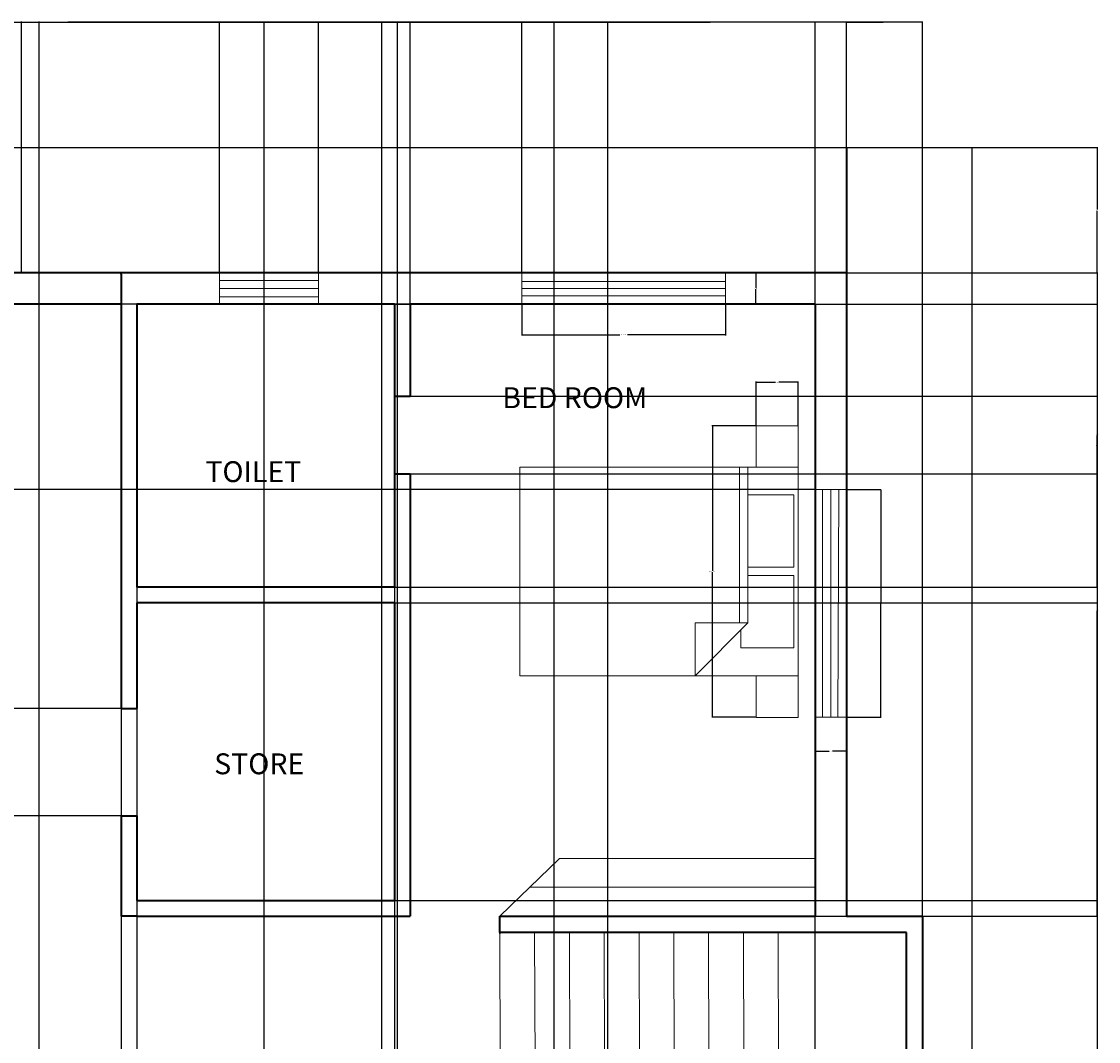
# Model space of a CAD drawing. Units: inches. Extents: x 2621 to 3621, y 1701 to 2465.
# Tile 4 of 6: x 2780 to 3090, y 2169 to 2462. Entities that reach past the tile are written whole.
import ezdxf

# ---------------------------------------------------------------- set-up
doc = ezdxf.new("R2010")
doc.units = ezdxf.units.IN
for name, color, linetype, lineweight in [('A-ANNO-DIMS', 2, 'Continuous', 18), ('A-AREA-IDEN', 7, 'Continuous', 18), ('A-FLOR-CASE', 32, 'Continuous', 18), ('A-FLOR-STRS', 30, 'Continuous', 18), ('A-FURN', 8, 'Continuous', 18), ('A-GLAZ', 4, 'Continuous', 18), ('A-WALL', 7, 'Continuous', 35), ('C-PROP', 8, 'Continuous', 25)]:
    doc.layers.add(name, color=color, linetype=linetype, lineweight=lineweight)
doc.styles.get("Standard").update_dxf_attribs({"font": 'arial.ttf'})
doc.dimstyles.get("Standard").update_dxf_attribs({"dimtxt": 0.18, "dimasz": 0.18, "dimexe": 0.18, "dimexo": 0.0625, "dimgap": 0.09, "dimtad": 0, "dimtih": 1, "dimtoh": 1, "dimdec": 4, "dimzin": 0, "dimdsep": 46, "dimtxsty": 'Standard', "dimcen": 0.09, "dimadec": 0, "dimazin": 0, "dimtfac": 1, "dimtdec": 4, "dimtofl": 0, "dimtmove": 0, "dimatfit": 3, "dimfxl": 1, "dimtolj": 1, "dimtzin": 0, "dimarcsym": 0})

# ---------------------------------------------------------------- blocks, each defined once
blk = doc.blocks.new('Bed - Queen')
for p, q in [((0, -80.00003), (0, 0)), ((0, 0), (59.99999, 0)), ((59.99999, 0), (59.99999, -80.00003)), ((7.99999, -1.2), (28.79998, -1.2)), ((7.99999, -14.4), (7.99999, -1.2)), ((28.79998, -1.2), (28.79998, -14.4)), ((31.19999, -1.2), (51.99999, -1.2)), ((31.19999, -14.4), (31.19999, -1.2)), ((51.99999, -1.2), (51.99999, -16.4)), ((0, -14.4), (44.8, -14.4)), ((59.99999, -29.6), (44.8, -14.4)), ((44.8, -14.4), (44.8, -29.6)), ((44.8, -16.8), (0, -16.8)), ((51.99999, -16.4), (46.79936, -16.4)), ((44.8, -29.6), (59.99999, -29.6)), ((59.99999, -80.00003), (0, -80.00003))]:
    blk.add_line(p, q)
blk = doc.blocks.new('LOT-33X57')
for p, q in [((0, 684), (396, 684)), ((396, 684), (396, 0))]:
    blk.add_line(p, q)
blk = doc.blocks.new('STAIR-RETURN-FLIGHT')
for p, q in [((30.25, 0.09), (30, 86.67)), ((40.25, 0.12), (40, 86.7)), ((50.25, 0.15), (50, 86.73)), ((60.25, 0.18), (60, 86.76)), ((70.25, 0.2), (70, 86.79)), ((80.25, 0.23), (80, 86.82)), ((0.25, 0), (0, 86.58)), ((10.25, 0.03), (10, 86.61)), ((20.25, 0.06), (20, 86.64)), ((6.51, 44.03), (0.13, 44.03)), ((79.82, 44.03), (6.51, 44.03)), ((79.82, 44.03), (80.13, 44.03)), ((6.51, 43.03), (0.13, 43.03)), ((79.82, 43.03), (6.51, 43.03)), ((79.82, 43.03), (80.13, 43.03)), ((70.59, 0.23), (70.59, 0.06))]:
    blk.add_line(p, q)
blk = doc.blocks.new('WIN-65_41')
for p, q in [((2.06, 65.41), (2.06, 0)), ((4.5, 65.41), (4.5, 0)), ((6.45, 0), (6.74, 65.41))]:
    blk.add_line(p, q)
blk.add_lwpolyline([(0, 65.41), (9, 65.41), (9, 0), (0, 0)], close=True)
blk = doc.blocks.new('WIN-58_50')
for p, q in [((0, 6.55), (58.5, 6.55)), ((0, 4.5), (58.5, 4.5)), ((0, 2.36), (58.5, 2.36))]:
    blk.add_line(p, q)
blk.add_lwpolyline([(0, 9), (58.5, 9), (58.5, 0), (0, 0)], close=True)
blk = doc.blocks.new('CASEWORK-BEDROOM-WALL-UNIT')
for p, q in [((0, 0), (17.18, 16.58)), ((17.18, 16.58), (90.65, 16.58)), ((8.59, 8.29), (90.65, 8.29))]:
    blk.add_line(p, q)
blk = doc.blocks.new('FURN-BEDSIDE-PAIR')
for points in [[(12, 71.92), (0, 71.92), (0, 83.71), (12, 83.71)], [(12, 11.92), (0, 11.92), (0, 0), (12, 0)]]:
    blk.add_lwpolyline(points, close=True)
blk = doc.blocks.new('*D21')
at = {"layer": 'A-ANNO-DIMS', "color": 0, "lineweight": -2, "transparency": 16777216}
for p, q in [((3017.58, 2327.19), (3027.51, 2327.19)), ((3027.33, 2327.01), (3027.33, 2294.66)), ((3027.33, 2261.96), (3027.33, 2294.3)), ((3017.58, 2261.78), (3027.51, 2261.78))]:
    blk.add_line(p, q, dxfattribs=at)
at = {"layer": 'A-ANNO-DIMS', "color": 0, "transparency": 16777216}
for points in [[(3027.3, 2327.01), (3027.36, 2327.01), (3027.33, 2327.19)], [(3027.3, 2261.96), (3027.36, 2261.96), (3027.33, 2261.78)]]:
    blk.add_solid(points, dxfattribs=at)
at = {"layer": 'Defpoints', "color": 0, "transparency": 16777216}
for p in [(3017.52, 2327.19), (3027.33, 2327.19), (3017.52, 2261.78)]:
    blk.add_point(p, dxfattribs=at)
at = {"layer": 'A-ANNO-DIMS', "color": 0, "transparency": 16777216, "insert": (3027.33, 2294.48), "char_height": 0.18, "attachment_point": 5}
blk.add_mtext('\\A1;WINDOW 65 TYP.', dxfattribs=at)
blk = doc.blocks.new('*D22')
at = {"layer": 'A-ANNO-DIMS', "color": 0, "lineweight": -2, "transparency": 16777216}
for p, q in [((3008.52, 2261.71), (3008.52, 2251.78)), ((3017.52, 2261.71), (3017.52, 2251.78)), ((3008.7, 2251.96), (3012.56, 2251.96)), ((3017.34, 2251.96), (3013.48, 2251.96))]:
    blk.add_line(p, q, dxfattribs=at)
at = {"layer": 'A-ANNO-DIMS', "color": 0, "transparency": 16777216}
for points in [[(3008.7, 2251.99), (3008.7, 2251.93), (3008.52, 2251.96)], [(3017.34, 2251.99), (3017.34, 2251.93), (3017.52, 2251.96)]]:
    blk.add_solid(points, dxfattribs=at)
at = {"layer": 'Defpoints', "color": 0, "transparency": 16777216}
for p in [(3008.52, 2261.78), (3017.52, 2261.78), (3017.52, 2251.96)]:
    blk.add_point(p, dxfattribs=at)
at = {"layer": 'A-ANNO-DIMS', "color": 0, "transparency": 16777216, "insert": (3013.02, 2251.96), "char_height": 0.18, "attachment_point": 5}
blk.add_mtext('\\A1;9 TYP.', dxfattribs=at)
blk = doc.blocks.new('*D25')
at = {"layer": 'A-ANNO-DIMS', "color": 0, "lineweight": -2, "transparency": 16777216}
for p, q in [((2924.2, 2380.34), (2924.2, 2371.45)), ((2982.7, 2380.34), (2982.7, 2371.45)), ((2924.38, 2371.63), (2952.33, 2371.63)), ((2982.52, 2371.63), (2954.57, 2371.63))]:
    blk.add_line(p, q, dxfattribs=at)
at = {"layer": 'A-ANNO-DIMS', "color": 0, "transparency": 16777216}
for points in [[(2924.38, 2371.66), (2924.38, 2371.6), (2924.2, 2371.63)], [(2982.52, 2371.66), (2982.52, 2371.6), (2982.7, 2371.63)]]:
    blk.add_solid(points, dxfattribs=at)
at = {"layer": 'Defpoints', "color": 0, "transparency": 16777216}
for p in [(2924.2, 2380.4), (2982.7, 2380.4), (2982.7, 2371.63)]:
    blk.add_point(p, dxfattribs=at)
at = {"layer": 'A-ANNO-DIMS', "color": 0, "transparency": 16777216, "insert": (2953.45, 2371.63), "char_height": 0.18, "attachment_point": 5}
blk.add_mtext('\\A1;WINDOW 59 TYP.', dxfattribs=at)
blk = doc.blocks.new('*D26')
at = {"layer": 'A-ANNO-DIMS', "color": 0, "lineweight": -2, "transparency": 16777216}
for p, q in [((2982.76, 2389.4), (2991.66, 2389.4)), ((2991.48, 2389.22), (2991.48, 2385.08)), ((2991.48, 2380.58), (2991.48, 2384.72)), ((2982.76, 2380.4), (2991.66, 2380.4))]:
    blk.add_line(p, q, dxfattribs=at)
at = {"layer": 'A-ANNO-DIMS', "color": 0, "transparency": 16777216}
for points in [[(2991.45, 2389.22), (2991.51, 2389.22), (2991.48, 2389.4)], [(2991.45, 2380.58), (2991.51, 2380.58), (2991.48, 2380.4)]]:
    blk.add_solid(points, dxfattribs=at)
at = {"layer": 'Defpoints', "color": 0, "transparency": 16777216}
for p in [(2982.7, 2389.4), (2991.48, 2389.4), (2982.7, 2380.4)]:
    blk.add_point(p, dxfattribs=at)
at = {"layer": 'A-ANNO-DIMS', "color": 0, "transparency": 16777216, "insert": (2991.48, 2384.9), "char_height": 0.18, "attachment_point": 5}
blk.add_mtext('\\A1;9 TYP.', dxfattribs=at)
blk = doc.blocks.new('*D29')
at = {"layer": 'A-ANNO-DIMS', "color": 0, "lineweight": -2, "transparency": 16777216}
for p, q in [((2991.52, 2345.41), (2978.84, 2345.41)), ((2979.02, 2345.23), (2979.02, 2303.74)), ((2979.02, 2261.88), (2979.02, 2303.37)), ((2991.52, 2261.7), (2978.84, 2261.7))]:
    blk.add_line(p, q, dxfattribs=at)
at = {"layer": 'A-ANNO-DIMS', "color": 0, "transparency": 16777216}
for points in [[(2978.99, 2345.23), (2979.05, 2345.23), (2979.02, 2345.41)], [(2978.99, 2261.88), (2979.05, 2261.88), (2979.02, 2261.7)]]:
    blk.add_solid(points, dxfattribs=at)
at = {"layer": 'Defpoints', "color": 0, "transparency": 16777216}
for p in [(2979.02, 2345.41), (2991.58, 2345.41), (2991.58, 2261.7)]:
    blk.add_point(p, dxfattribs=at)
at = {"layer": 'A-ANNO-DIMS', "color": 0, "transparency": 16777216, "insert": (2979.02, 2303.55), "char_height": 0.18, "attachment_point": 5}
blk.add_mtext('\\A1;BEDSIDE PAIR 84 TYP.', dxfattribs=at)
blk = doc.blocks.new('*D30')
at = {"layer": 'A-ANNO-DIMS', "color": 0, "lineweight": -2, "transparency": 16777216}
for p, q in [((2991.58, 2345.47), (2991.58, 2358.15)), ((2991.76, 2357.97), (2997.06, 2357.97)), ((3003.4, 2357.97), (2998.1, 2357.97)), ((3003.58, 2345.47), (3003.58, 2358.15))]:
    blk.add_line(p, q, dxfattribs=at)
at = {"layer": 'A-ANNO-DIMS', "color": 0, "transparency": 16777216}
for points in [[(2991.76, 2358), (2991.76, 2357.94), (2991.58, 2357.97)], [(3003.4, 2358), (3003.4, 2357.94), (3003.58, 2357.97)]]:
    blk.add_solid(points, dxfattribs=at)
at = {"layer": 'Defpoints', "color": 0, "transparency": 16777216}
for p in [(3003.58, 2357.97), (2991.58, 2345.41), (3003.58, 2345.41)]:
    blk.add_point(p, dxfattribs=at)
at = {"layer": 'A-ANNO-DIMS', "color": 0, "transparency": 16777216, "insert": (2997.58, 2357.97), "char_height": 0.18, "attachment_point": 5}
blk.add_mtext('\\A1;12 TYP.', dxfattribs=at)
blk = doc.blocks.new('*D37')
at = {"layer": 'A-ANNO-DIMS', "color": 0, "lineweight": -2, "transparency": 16777216}
for p, q in [((2693.52, 2425.46), (2693.52, 2461.61)), ((2693.7, 2461.43), (2865.98, 2461.43)), ((3039.19, 2461.43), (2866.91, 2461.43)), ((3039.37, 2204.63), (3039.37, 2461.61))]:
    blk.add_line(p, q, dxfattribs=at)
at = {"layer": 'A-ANNO-DIMS', "color": 0, "transparency": 16777216}
for points in [[(2693.7, 2461.46), (2693.7, 2461.4), (2693.52, 2461.43)], [(3039.19, 2461.46), (3039.19, 2461.4), (3039.37, 2461.43)]]:
    blk.add_solid(points, dxfattribs=at)
at = {"layer": 'Defpoints', "color": 0, "transparency": 16777216}
for p in [(3039.37, 2461.43), (2693.52, 2425.4), (3039.37, 2204.57)]:
    blk.add_point(p, dxfattribs=at)
at = {"layer": 'A-ANNO-DIMS', "color": 0, "transparency": 16777216, "insert": (2866.44, 2461.43), "char_height": 0.18, "attachment_point": 5}
blk.add_mtext('\\A1;345.85', dxfattribs=at)
blk = doc.blocks.new('*D38')
at = {"layer": 'A-ANNO-DIMS', "color": 0, "lineweight": -2, "transparency": 16777216}
for p, q in [((3017.58, 2389.4), (3089.72, 2389.4)), ((3089.54, 2389.22), (3089.54, 2083.58)), ((3089.54, 1777.58), (3089.54, 2083.22)), ((3017.58, 1777.4), (3089.72, 1777.4))]:
    blk.add_line(p, q, dxfattribs=at)
at = {"layer": 'A-ANNO-DIMS', "color": 0, "transparency": 16777216}
for points in [[(3089.51, 2389.22), (3089.57, 2389.22), (3089.54, 2389.4)], [(3089.51, 1777.58), (3089.57, 1777.58), (3089.54, 1777.4)]]:
    blk.add_solid(points, dxfattribs=at)
at = {"layer": 'Defpoints', "color": 0, "transparency": 16777216}
for p in [(3017.52, 2389.4), (3089.54, 2389.4), (3017.52, 1777.4)]:
    blk.add_point(p, dxfattribs=at)
at = {"layer": 'A-ANNO-DIMS', "color": 0, "transparency": 16777216, "insert": (3089.54, 2083.4), "char_height": 0.18, "attachment_point": 5}
blk.add_mtext('\\A1;612', dxfattribs=at)
blk = doc.blocks.new('*D41')
at = {"layer": 'A-ANNO-DIMS', "color": 0, "lineweight": -2, "transparency": 16777216}
for p, q in [((2693.58, 2425.4), (3089.72, 2425.4)), ((3089.54, 2425.22), (3089.54, 2407.58)), ((3089.54, 2389.58), (3089.54, 2407.22)), ((2693.58, 2389.4), (3089.72, 2389.4))]:
    blk.add_line(p, q, dxfattribs=at)
at = {"layer": 'A-ANNO-DIMS', "color": 0, "transparency": 16777216}
for points in [[(3089.51, 2425.22), (3089.57, 2425.22), (3089.54, 2425.4)], [(3089.51, 2389.58), (3089.57, 2389.58), (3089.54, 2389.4)]]:
    blk.add_solid(points, dxfattribs=at)
at = {"layer": 'Defpoints', "color": 0, "transparency": 16777216}
for p in [(2693.52, 2425.4), (2693.52, 2389.4), (3089.54, 2389.4)]:
    blk.add_point(p, dxfattribs=at)
at = {"layer": 'A-ANNO-DIMS', "color": 0, "transparency": 16777216, "insert": (3089.54, 2407.4), "char_height": 0.18, "attachment_point": 5}
blk.add_mtext('\\A1;36', dxfattribs=at)
blk = doc.blocks.new('*D42')
at = {"layer": 'A-ANNO-DIMS', "color": 0, "lineweight": -2, "transparency": 16777216}
for p, q in [((2702.52, 2380.34), (2702.52, 1705.2)), ((2809.02, 2380.34), (2809.02, 1705.2)), ((2702.7, 1705.38), (2755.38, 1705.38)), ((2808.84, 1705.38), (2756.15, 1705.38))]:
    blk.add_line(p, q, dxfattribs=at)
at = {"layer": 'A-ANNO-DIMS', "color": 0, "transparency": 16777216}
for points in [[(2702.7, 1705.41), (2702.7, 1705.35), (2702.52, 1705.38)], [(2808.84, 1705.41), (2808.84, 1705.35), (2809.02, 1705.38)]]:
    blk.add_solid(points, dxfattribs=at)
at = {"layer": 'Defpoints', "color": 0, "transparency": 16777216}
for p in [(2702.52, 2380.4), (2809.02, 2380.4), (2809.02, 1705.38)]:
    blk.add_point(p, dxfattribs=at)
at = {"layer": 'A-ANNO-DIMS', "color": 0, "transparency": 16777216, "insert": (2755.77, 1705.38), "char_height": 0.18, "attachment_point": 5}
blk.add_mtext('\\A1;106.5', dxfattribs=at)
blk = doc.blocks.new('*D43')
at = {"layer": 'A-ANNO-DIMS', "color": 0, "lineweight": -2, "transparency": 16777216}
for p, q in [((2813.52, 2380.34), (2813.52, 1705.2)), ((2887.57, 2380.34), (2887.57, 1705.2)), ((2813.7, 1705.38), (2850.15, 1705.38)), ((2887.39, 1705.38), (2850.94, 1705.38))]:
    blk.add_line(p, q, dxfattribs=at)
at = {"layer": 'A-ANNO-DIMS', "color": 0, "transparency": 16777216}
for points in [[(2813.7, 1705.41), (2813.7, 1705.35), (2813.52, 1705.38)], [(2887.39, 1705.41), (2887.39, 1705.35), (2887.57, 1705.38)]]:
    blk.add_solid(points, dxfattribs=at)
at = {"layer": 'Defpoints', "color": 0, "transparency": 16777216}
for p in [(2813.52, 2380.4), (2887.57, 2380.4), (2887.57, 1705.38)]:
    blk.add_point(p, dxfattribs=at)
at = {"layer": 'A-ANNO-DIMS', "color": 0, "transparency": 16777216, "insert": (2850.55, 1705.38), "char_height": 0.18, "attachment_point": 5}
blk.add_mtext('\\A1;74.05', dxfattribs=at)
blk = doc.blocks.new('*D44')
at = {"layer": 'A-ANNO-DIMS', "color": 0, "lineweight": -2, "transparency": 16777216}
for p, q in [((2892.07, 2380.46), (2892.07, 2461.61)), ((2892.25, 2461.43), (2949.84, 2461.43)), ((3008.34, 2461.43), (2950.75, 2461.43)), ((3008.52, 2380.46), (3008.52, 2461.61))]:
    blk.add_line(p, q, dxfattribs=at)
at = {"layer": 'A-ANNO-DIMS', "color": 0, "transparency": 16777216}
for points in [[(2892.25, 2461.46), (2892.25, 2461.4), (2892.07, 2461.43)], [(3008.34, 2461.46), (3008.34, 2461.4), (3008.52, 2461.43)]]:
    blk.add_solid(points, dxfattribs=at)
at = {"layer": 'Defpoints', "color": 0, "transparency": 16777216}
for p in [(3008.52, 2461.43), (2892.07, 2380.4), (3008.52, 2380.4)]:
    blk.add_point(p, dxfattribs=at)
at = {"layer": 'A-ANNO-DIMS', "color": 0, "transparency": 16777216, "insert": (2950.3, 2461.43), "char_height": 0.18, "attachment_point": 5}
blk.add_mtext('\\A1;116.45', dxfattribs=at)
blk = doc.blocks.new('*D45')
at = {"layer": 'A-ANNO-DIMS', "color": 0, "lineweight": -2, "transparency": 16777216}
for p, q in [((2813.58, 2380.4), (3089.72, 2380.4)), ((3089.54, 2380.22), (3089.54, 2339.92)), ((3089.54, 2299.25), (3089.54, 2339.55)), ((2813.58, 2299.07), (3089.72, 2299.07))]:
    blk.add_line(p, q, dxfattribs=at)
at = {"layer": 'A-ANNO-DIMS', "color": 0, "transparency": 16777216}
for points in [[(3089.51, 2380.22), (3089.57, 2380.22), (3089.54, 2380.4)], [(3089.51, 2299.25), (3089.57, 2299.25), (3089.54, 2299.07)]]:
    blk.add_solid(points, dxfattribs=at)
at = {"layer": 'Defpoints', "color": 0, "transparency": 16777216}
for p in [(2813.52, 2380.4), (3089.54, 2380.4), (2813.52, 2299.07)]:
    blk.add_point(p, dxfattribs=at)
at = {"layer": 'A-ANNO-DIMS', "color": 0, "transparency": 16777216, "insert": (3089.54, 2339.74), "char_height": 0.18, "attachment_point": 5}
blk.add_mtext('\\A1;81.33', dxfattribs=at)
blk = doc.blocks.new('*D46')
at = {"layer": 'A-ANNO-DIMS', "color": 0, "lineweight": -2, "transparency": 16777216}
for p, q in [((2813.59, 2294.57), (3089.72, 2294.57)), ((3089.54, 2294.39), (3089.54, 2252)), ((3089.54, 2209.25), (3089.54, 2251.64)), ((2813.58, 2209.07), (3089.72, 2209.07))]:
    blk.add_line(p, q, dxfattribs=at)
at = {"layer": 'A-ANNO-DIMS', "color": 0, "transparency": 16777216}
for points in [[(3089.51, 2294.39), (3089.57, 2294.39), (3089.54, 2294.57)], [(3089.51, 2209.25), (3089.57, 2209.25), (3089.54, 2209.07)]]:
    blk.add_solid(points, dxfattribs=at)
at = {"layer": 'Defpoints', "color": 0, "transparency": 16777216}
for p in [(2813.53, 2294.57), (3089.54, 2294.57), (2813.52, 2209.07)]:
    blk.add_point(p, dxfattribs=at)
at = {"layer": 'A-ANNO-DIMS', "color": 0, "transparency": 16777216, "insert": (3089.54, 2251.82), "char_height": 0.18, "attachment_point": 5}
blk.add_mtext('\\A1;85.5', dxfattribs=at)
blk = doc.blocks.new('*D47')
at = {"layer": 'A-ANNO-DIMS', "color": 0, "lineweight": -2, "transparency": 16777216}
for p, q in [((3008.58, 2380.4), (3089.72, 2380.4)), ((3089.54, 2380.22), (3089.54, 2292.67)), ((3089.54, 2204.75), (3089.54, 2292.3)), ((3008.58, 2204.57), (3089.72, 2204.57))]:
    blk.add_line(p, q, dxfattribs=at)
at = {"layer": 'A-ANNO-DIMS', "color": 0, "transparency": 16777216}
for points in [[(3089.51, 2380.22), (3089.57, 2380.22), (3089.54, 2380.4)], [(3089.51, 2204.75), (3089.57, 2204.75), (3089.54, 2204.57)]]:
    blk.add_solid(points, dxfattribs=at)
at = {"layer": 'Defpoints', "color": 0, "transparency": 16777216}
for p in [(3008.52, 2380.4), (3089.54, 2380.4), (3008.52, 2204.57)]:
    blk.add_point(p, dxfattribs=at)
at = {"layer": 'A-ANNO-DIMS', "color": 0, "transparency": 16777216, "insert": (3089.54, 2292.49), "char_height": 0.18, "attachment_point": 5}
blk.add_mtext('\\A1;175.83', dxfattribs=at)
blk = doc.blocks.new('*D52')
at = {"layer": 'A-ANNO-DIMS', "color": 0, "lineweight": -2, "transparency": 16777216}
for p, q in [((2702.52, 1892.46), (2702.52, 2461.61)), ((2702.7, 2461.43), (2792.8, 2461.43)), ((2883.82, 2461.43), (2793.71, 2461.43)), ((2884, 1887.96), (2884, 2461.61))]:
    blk.add_line(p, q, dxfattribs=at)
at = {"layer": 'A-ANNO-DIMS', "color": 0, "transparency": 16777216}
for points in [[(2702.7, 2461.46), (2702.7, 2461.4), (2702.52, 2461.43)], [(2883.82, 2461.46), (2883.82, 2461.4), (2884, 2461.43)]]:
    blk.add_solid(points, dxfattribs=at)
at = {"layer": 'Defpoints', "color": 0, "transparency": 16777216}
for p in [(2884, 2461.43), (2702.52, 1892.4), (2884, 1887.9)]:
    blk.add_point(p, dxfattribs=at)
at = {"layer": 'A-ANNO-DIMS', "color": 0, "transparency": 16777216, "insert": (2793.26, 2461.43), "char_height": 0.18, "attachment_point": 5}
blk.add_mtext('\\A1;181.48', dxfattribs=at)
blk = doc.blocks.new('*D53')
at = {"layer": 'A-ANNO-DIMS', "color": 0, "lineweight": -2, "transparency": 16777216}
for p, q in [((2888.5, 1777.46), (2888.5, 2461.61)), ((2888.68, 2461.43), (2948.05, 2461.43)), ((3008.34, 2461.43), (2948.96, 2461.43)), ((3008.52, 1777.46), (3008.52, 2461.61))]:
    blk.add_line(p, q, dxfattribs=at)
at = {"layer": 'A-ANNO-DIMS', "color": 0, "transparency": 16777216}
for points in [[(2888.68, 2461.46), (2888.68, 2461.4), (2888.5, 2461.43)], [(3008.34, 2461.46), (3008.34, 2461.4), (3008.52, 2461.43)]]:
    blk.add_solid(points, dxfattribs=at)
at = {"layer": 'Defpoints', "color": 0, "transparency": 16777216}
for p in [(3008.52, 2461.43), (2888.5, 1777.4), (3008.52, 1777.4)]:
    blk.add_point(p, dxfattribs=at)
at = {"layer": 'A-ANNO-DIMS', "color": 0, "transparency": 16777216, "insert": (2948.51, 2461.43), "char_height": 0.18, "attachment_point": 5}
blk.add_mtext('\\A1;120.02', dxfattribs=at)
blk = doc.blocks.new('*D56')
at = {"layer": 'A-ANNO-DIMS', "color": 0, "lineweight": -2, "transparency": 16777216}
for p, q in [((2948.9, 2012.46), (2948.9, 2461.61)), ((2949.08, 2461.43), (2978.32, 2461.43)), ((3008.34, 2461.43), (2979.1, 2461.43)), ((3008.52, 2012.46), (3008.52, 2461.61))]:
    blk.add_line(p, q, dxfattribs=at)
at = {"layer": 'A-ANNO-DIMS', "color": 0, "transparency": 16777216}
for points in [[(2949.08, 2461.46), (2949.08, 2461.4), (2948.9, 2461.43)], [(3008.34, 2461.46), (3008.34, 2461.4), (3008.52, 2461.43)]]:
    blk.add_solid(points, dxfattribs=at)
at = {"layer": 'Defpoints', "color": 0, "transparency": 16777216}
for p in [(3008.52, 2461.43), (2948.9, 2012.4), (3008.52, 2012.4)]:
    blk.add_point(p, dxfattribs=at)
at = {"layer": 'A-ANNO-DIMS', "color": 0, "transparency": 16777216, "insert": (2978.71, 2461.43), "char_height": 0.18, "attachment_point": 5}
blk.add_mtext('\\A1;59.62', dxfattribs=at)
blk = doc.blocks.new('*D59')
at = {"layer": 'A-ANNO-DIMS', "color": 0, "lineweight": -2, "transparency": 16777216}
for p, q in [((2933.47, 2007.96), (2933.47, 2461.61)), ((2933.65, 2461.43), (2970.6, 2461.43)), ((3008.34, 2461.43), (2971.39, 2461.43)), ((3008.52, 2007.96), (3008.52, 2461.61))]:
    blk.add_line(p, q, dxfattribs=at)
at = {"layer": 'A-ANNO-DIMS', "color": 0, "transparency": 16777216}
for points in [[(2933.65, 2461.46), (2933.65, 2461.4), (2933.47, 2461.43)], [(3008.34, 2461.46), (3008.34, 2461.4), (3008.52, 2461.43)]]:
    blk.add_solid(points, dxfattribs=at)
at = {"layer": 'Defpoints', "color": 0, "transparency": 16777216}
for p in [(3008.52, 2461.43), (2933.47, 2007.9), (3008.52, 2007.9)]:
    blk.add_point(p, dxfattribs=at)
at = {"layer": 'A-ANNO-DIMS', "color": 0, "transparency": 16777216, "insert": (2971, 2461.43), "char_height": 0.18, "attachment_point": 5}
blk.add_mtext('\\A1;75.04', dxfattribs=at)
blk = doc.blocks.new('*D60')
at = {"layer": 'A-ANNO-DIMS', "color": 0, "lineweight": -2, "transparency": 16777216}
for p, q in [((3017.52, 2204.63), (3017.52, 2461.61)), ((3017.7, 2461.43), (3028.05, 2461.43)), ((3039.19, 2461.43), (3028.84, 2461.43)), ((3039.37, 2204.63), (3039.37, 2461.61))]:
    blk.add_line(p, q, dxfattribs=at)
at = {"layer": 'A-ANNO-DIMS', "color": 0, "transparency": 16777216}
for points in [[(3017.7, 2461.46), (3017.7, 2461.4), (3017.52, 2461.43)], [(3039.19, 2461.46), (3039.19, 2461.4), (3039.37, 2461.43)]]:
    blk.add_solid(points, dxfattribs=at)
at = {"layer": 'Defpoints', "color": 0, "transparency": 16777216}
for p in [(3039.37, 2461.43), (3017.52, 2204.57), (3039.37, 2204.57)]:
    blk.add_point(p, dxfattribs=at)
at = {"layer": 'A-ANNO-DIMS', "color": 0, "transparency": 16777216, "insert": (3028.44, 2461.43), "char_height": 0.18, "attachment_point": 5}
blk.add_mtext('\\A1;21.85', dxfattribs=at)
blk = doc.blocks.new('*D61')
at = {"layer": 'A-ANNO-DIMS', "color": 0, "lineweight": -2, "transparency": 16777216}
for p, q in [((2785.46, 1857.23), (2785.46, 2461.61)), ((2785.64, 2461.43), (2834.33, 2461.43)), ((2883.82, 2461.43), (2835.12, 2461.43)), ((2884, 1857.23), (2884, 2461.61))]:
    blk.add_line(p, q, dxfattribs=at)
at = {"layer": 'A-ANNO-DIMS', "color": 0, "transparency": 16777216}
for points in [[(2785.64, 2461.46), (2785.64, 2461.4), (2785.46, 2461.43)], [(2883.82, 2461.46), (2883.82, 2461.4), (2884, 2461.43)]]:
    blk.add_solid(points, dxfattribs=at)
at = {"layer": 'Defpoints', "color": 0, "transparency": 16777216}
for p in [(2884, 2461.43), (2785.46, 1857.17), (2884, 1857.17)]:
    blk.add_point(p, dxfattribs=at)
at = {"layer": 'A-ANNO-DIMS', "color": 0, "transparency": 16777216, "insert": (2834.73, 2461.43), "char_height": 0.18, "attachment_point": 5}
blk.add_mtext('\\A1;98.54', dxfattribs=at)
blk = doc.blocks.new('*D82')
at = {"layer": 'A-ANNO-DIMS', "color": 0, "lineweight": -2, "transparency": 16777216}
for p, q in [((2780.41, 2389.46), (2780.41, 2461.61)), ((2780.59, 2461.43), (2808.48, 2461.43)), ((2837.15, 2461.43), (2809.26, 2461.43)), ((2837.33, 2389.46), (2837.33, 2461.61))]:
    blk.add_line(p, q, dxfattribs=at)
at = {"layer": 'A-ANNO-DIMS', "color": 0, "transparency": 16777216}
for points in [[(2780.59, 2461.46), (2780.59, 2461.4), (2780.41, 2461.43)], [(2837.15, 2461.46), (2837.15, 2461.4), (2837.33, 2461.43)]]:
    blk.add_solid(points, dxfattribs=at)
at = {"layer": 'Defpoints', "color": 0, "transparency": 16777216}
for p in [(2837.33, 2461.43), (2780.41, 2389.4), (2837.33, 2389.4)]:
    blk.add_point(p, dxfattribs=at)
at = {"layer": 'A-ANNO-DIMS', "color": 0, "transparency": 16777216, "insert": (2808.87, 2461.43), "char_height": 0.18, "attachment_point": 5}
blk.add_mtext('\\A1;56.92', dxfattribs=at)
blk = doc.blocks.new('*D83')
at = {"layer": 'A-ANNO-DIMS', "color": 0, "lineweight": -2, "transparency": 16777216}
for p, q in [((2837.33, 2389.46), (2837.33, 2461.61)), ((2837.51, 2461.43), (2851.15, 2461.43)), ((2865.58, 2461.43), (2851.94, 2461.43)), ((2865.76, 2389.46), (2865.76, 2461.61))]:
    blk.add_line(p, q, dxfattribs=at)
at = {"layer": 'A-ANNO-DIMS', "color": 0, "transparency": 16777216}
for points in [[(2837.51, 2461.46), (2837.51, 2461.4), (2837.33, 2461.43)], [(2865.58, 2461.46), (2865.58, 2461.4), (2865.76, 2461.43)]]:
    blk.add_solid(points, dxfattribs=at)
at = {"layer": 'Defpoints', "color": 0, "transparency": 16777216}
for p in [(2865.76, 2461.43), (2837.33, 2389.4), (2865.76, 2389.4)]:
    blk.add_point(p, dxfattribs=at)
at = {"layer": 'A-ANNO-DIMS', "color": 0, "transparency": 16777216, "insert": (2851.54, 2461.43), "char_height": 0.18, "attachment_point": 5}
blk.add_mtext('\\A1;28.43', dxfattribs=at)
blk = doc.blocks.new('*D84')
at = {"layer": 'A-ANNO-DIMS', "color": 0, "lineweight": -2, "transparency": 16777216}
for p, q in [((2865.76, 2389.46), (2865.76, 2461.61)), ((2865.94, 2461.43), (2894.58, 2461.43)), ((2924.02, 2461.43), (2895.37, 2461.43)), ((2924.2, 2389.46), (2924.2, 2461.61))]:
    blk.add_line(p, q, dxfattribs=at)
at = {"layer": 'A-ANNO-DIMS', "color": 0, "transparency": 16777216}
for points in [[(2865.94, 2461.46), (2865.94, 2461.4), (2865.76, 2461.43)], [(2924.02, 2461.46), (2924.02, 2461.4), (2924.2, 2461.43)]]:
    blk.add_solid(points, dxfattribs=at)
at = {"layer": 'Defpoints', "color": 0, "transparency": 16777216}
for p in [(2924.2, 2461.43), (2865.76, 2389.4), (2924.2, 2389.4)]:
    blk.add_point(p, dxfattribs=at)
at = {"layer": 'A-ANNO-DIMS', "color": 0, "transparency": 16777216, "insert": (2894.98, 2461.43), "char_height": 0.18, "attachment_point": 5}
blk.add_mtext('\\A1;58.44', dxfattribs=at)
blk = doc.blocks.new('*D91')
at = {"layer": 'A-ANNO-DIMS', "color": 0, "lineweight": -2, "transparency": 16777216}
for p, q in [((3008.46, 2380.4), (2621.31, 2380.4)), ((2621.49, 2380.22), (2621.49, 2353.98)), ((2621.49, 2327.37), (2621.49, 2353.61)), ((3008.46, 2327.19), (2621.31, 2327.19))]:
    blk.add_line(p, q, dxfattribs=at)
at = {"layer": 'A-ANNO-DIMS', "color": 0, "transparency": 16777216}
for points in [[(2621.46, 2380.22), (2621.52, 2380.22), (2621.49, 2380.4)], [(2621.46, 2327.37), (2621.52, 2327.37), (2621.49, 2327.19)]]:
    blk.add_solid(points, dxfattribs=at)
at = {"layer": 'Defpoints', "color": 0, "transparency": 16777216}
for p in [(2621.49, 2380.4), (3008.52, 2380.4), (3008.52, 2327.19)]:
    blk.add_point(p, dxfattribs=at)
at = {"layer": 'A-ANNO-DIMS', "color": 0, "transparency": 16777216, "insert": (2621.49, 2353.79), "char_height": 0.18, "attachment_point": 5}
blk.add_mtext('\\A1;53.22', dxfattribs=at)
blk = doc.blocks.new('*D100')
at = {"layer": 'A-ANNO-DIMS', "color": 0, "lineweight": -2, "transparency": 16777216}
for p, q in [((2850.13, 2113.32), (2850.13, 2461.61)), ((2850.31, 2461.43), (2866.67, 2461.43)), ((2883.82, 2461.43), (2867.45, 2461.43)), ((2884, 2113.32), (2884, 2461.61))]:
    blk.add_line(p, q, dxfattribs=at)
at = {"layer": 'A-ANNO-DIMS', "color": 0, "transparency": 16777216}
for points in [[(2850.31, 2461.46), (2850.31, 2461.4), (2850.13, 2461.43)], [(2883.82, 2461.46), (2883.82, 2461.4), (2884, 2461.43)]]:
    blk.add_solid(points, dxfattribs=at)
at = {"layer": 'Defpoints', "color": 0, "transparency": 16777216}
for p in [(2884, 2461.43), (2850.13, 2113.25), (2884, 2113.25)]:
    blk.add_point(p, dxfattribs=at)
at = {"layer": 'A-ANNO-DIMS', "color": 0, "transparency": 16777216, "insert": (2867.06, 2461.43), "char_height": 0.18, "attachment_point": 5}
blk.add_mtext('\\A1;33.87', dxfattribs=at)
blk = doc.blocks.new('*D101')
at = {"layer": 'A-ANNO-DIMS', "color": 0, "lineweight": -2, "transparency": 16777216}
for p, q in [((2808.96, 2264.26), (2621.31, 2264.26)), ((2621.49, 2264.08), (2621.49, 2248.99)), ((2621.49, 2233.55), (2621.49, 2248.63)), ((2808.96, 2233.37), (2621.31, 2233.37))]:
    blk.add_line(p, q, dxfattribs=at)
at = {"layer": 'A-ANNO-DIMS', "color": 0, "transparency": 16777216}
for points in [[(2621.46, 2264.08), (2621.52, 2264.08), (2621.49, 2264.26)], [(2621.46, 2233.55), (2621.52, 2233.55), (2621.49, 2233.37)]]:
    blk.add_solid(points, dxfattribs=at)
at = {"layer": 'Defpoints', "color": 0, "transparency": 16777216}
for p in [(2621.49, 2264.26), (2809.02, 2264.26), (2809.02, 2233.37)]:
    blk.add_point(p, dxfattribs=at)
at = {"layer": 'A-ANNO-DIMS', "color": 0, "transparency": 16777216, "insert": (2621.49, 2248.81), "char_height": 0.18, "attachment_point": 5}
blk.add_mtext('\\A1;30.896', dxfattribs=at)
blk = doc.blocks.new('*D102')
at = {"layer": 'A-ANNO-DIMS', "color": 0, "lineweight": -2, "transparency": 16777216}
for p, q in [((2892.14, 2353.99), (3089.72, 2353.99)), ((3089.54, 2353.81), (3089.54, 2343.01)), ((3089.54, 2331.85), (3089.54, 2342.65)), ((2892.14, 2331.67), (3089.72, 2331.67))]:
    blk.add_line(p, q, dxfattribs=at)
at = {"layer": 'A-ANNO-DIMS', "color": 0, "transparency": 16777216}
for points in [[(3089.51, 2353.81), (3089.57, 2353.81), (3089.54, 2353.99)], [(3089.51, 2331.85), (3089.57, 2331.85), (3089.54, 2331.67)]]:
    blk.add_solid(points, dxfattribs=at)
at = {"layer": 'Defpoints', "color": 0, "transparency": 16777216}
for p in [(2892.07, 2353.99), (3089.54, 2353.99), (2892.07, 2331.67)]:
    blk.add_point(p, dxfattribs=at)
at = {"layer": 'A-ANNO-DIMS', "color": 0, "transparency": 16777216, "insert": (3089.54, 2342.83), "char_height": 0.18, "attachment_point": 5}
blk.add_mtext('\\A1;22.324', dxfattribs=at)

msp = doc.modelspace()

# ---------------------------------------------------------------- linework, layer by layer
at = {"layer": 'A-GLAZ'}
for p, q in [((2837.328, 2387.2101), (2865.7552, 2387.2101)), ((2837.328, 2382.5213), (2865.7552, 2382.5213))]:
    msp.add_line(p, q, dxfattribs=at)
for points in [[(2837.328, 2389.4015), (2865.7552, 2389.4015), (2865.7552, 2380.4015), (2837.328, 2380.4015)], [(2837.328, 2384.9015), (2865.7552, 2384.9015), (2865.7552, 2384.9015), (2837.328, 2384.9015)]]:
    msp.add_lwpolyline(points, close=True, dxfattribs=at)
at = {"layer": 'A-WALL'}
for p, q in [((3017.5184, 2425.4015), (3017.5184, 2204.5707)), ((3017.5184, 2389.4015), (2693.5184, 2389.4015)), ((2809.0179, 2389.0707), (2809.0179, 2389.4015)), ((2809.0179, 2389.0707), (2809.0179, 2264.2608)), ((2809.0179, 2380.4015), (2702.5184, 2380.4015)), ((2813.5179, 2380.4015), (2813.5179, 2299.0707)), ((2887.5726, 2380.4015), (2813.5179, 2380.4015)), ((2887.5726, 2380.4015), (2887.5726, 2299.2361)), ((3008.5184, 2380.4015), (2892.0726, 2380.4015)), ((2892.0726, 2380.4015), (2892.0726, 2353.9943)), ((3008.5184, 2380.4015), (3008.5184, 2204.5707)), ((2887.5726, 2353.9943), (2892.0726, 2353.9943)), ((2887.5726, 2331.6701), (2892.0726, 2331.6701)), ((2892.0726, 2331.6701), (2892.0726, 2209.0707)), ((2887.5726, 2299.2361), (2813.5179, 2299.0707)), ((2887.5827, 2294.7361), (2813.528, 2294.5707)), ((2813.528, 2294.5707), (2813.528, 2264.2608)), ((2887.5726, 2294.7361), (2887.5726, 2209.0707)), ((2809.0179, 2264.2608), (2813.528, 2264.2608)), ((2809.0179, 2233.3652), (2813.528, 2233.3652)), ((2809.0179, 2233.3652), (2809.0179, 2209.0707)), ((2813.528, 2233.3652), (2813.528, 2209.0707)), ((2809.0179, 2209.0707), (2809.0179, 2204.5707)), ((2813.5179, 2209.0707), (2887.5726, 2209.0707)), ((2892.0726, 2209.0707), (2892.0726, 2204.5707)), ((2813.5179, 2204.5707), (2809.0179, 2204.5707)), ((2813.5179, 2204.5707), (2892.0726, 2204.5707)), ((2917.8715, 2204.5707), (3008.5184, 2204.5707)), ((2917.8715, 2199.8382), (2917.8715, 2204.5707)), ((3017.5184, 2204.5707), (3039.3697, 2204.5707)), ((3039.3697, 2204.5707), (3039.3697, 2108.7527)), ((2924.38, 2199.8382), (2917.8715, 2199.8382)), ((2917.8715, 2199.8382), (2917.8715, 2199.8382)), ((2917.8715, 2199.8382), (2917.8715, 2199.604)), ((3034.7824, 2199.8382), (2924.38, 2199.8382)), ((3034.7824, 2113.2527), (3034.7824, 2199.8382))]:
    msp.add_line(p, q, dxfattribs=at)

# ---------------------------------------------------------------- block references
at = {"layer": 'A-FLOR-CASE'}
msp.add_blockref('CASEWORK-BEDROOM-WALL-UNIT', (2917.871, 2204.571), dxfattribs=at)
at = {"layer": 'A-FLOR-STRS'}
msp.add_blockref('STAIR-RETURN-FLIGHT', (2917.871, 2113.019), dxfattribs=at)
at = {"layer": 'A-FURN'}
msp.add_blockref('FURN-BEDSIDE-PAIR', (2991.578, 2261.696), dxfattribs=at)
at = {"layer": 'A-FURN', "rotation": 270}
msp.add_blockref('Bed - Queen', (3003.5782, 2333.6172), dxfattribs=at)
at = {"layer": 'A-GLAZ'}
for name, p in [('WIN-58_50', (2924.198, 2380.402)), ('WIN-65_41', (3008.518, 2261.775))]:
    msp.add_blockref(name, p, dxfattribs=at)
at = {"layer": 'C-PROP'}
msp.add_blockref('LOT-33X57', (2657.518, 1741.402), dxfattribs=at)

# ---------------------------------------------------------------- texts
at = {"layer": 'A-AREA-IDEN', "char_height": 6, "attachment_point": 1}
for s, width, insert in [('BED ROOM ', 51.297978, (2918.5804, 2356.5281)), ('TOILET', 19.625331, (2833.2377, 2335.2762)), ('STORE', 19.625331, (2835.7842, 2251.3439))]:
    msp.add_mtext_dynamic_manual_height_columns(s, width=width, gutter_width=12.5, heights=[0], dxfattribs=dict(at, insert=insert))

# ---------------------------------------------------------------- dimensions: what is measured, and where the dimension line sits
at = {"layer": 'A-ANNO-DIMS'}
for base, p1, p2, override, picture, middle in [((3039.3697, 2461.427), (2693.5184, 2425.4015), (3039.3697, 2204.5707), {"dimdec": 2, "dimlfac": 1, "dimrnd": 0, "dimzin": 0, "dimdsep": 46, "dimlunit": 2}, '*D37', (2866.444, 2461.427)), ((2883.995, 2461.427), (2702.5184, 1892.3987), (2883.995, 1887.8987), {"dimdec": 2, "dimlfac": 1, "dimrnd": 0, "dimzin": 0, "dimdsep": 46, "dimlunit": 2}, '*D52', (2793.2567, 2461.427)), ((2837.328, 2461.427), (2780.4086, 2389.4015), (2837.328, 2389.4015), {"dimdec": 2, "dimlfac": 1, "dimrnd": 0, "dimzin": 0, "dimdsep": 46, "dimlunit": 2}, '*D82', (2808.8683, 2461.427)), ((2883.995, 2461.427), (2785.4592, 1857.1678), (2883.995, 1857.1678), {"dimdec": 2, "dimlfac": 1, "dimrnd": 0, "dimzin": 0, "dimdsep": 46, "dimlunit": 2}, '*D61', (2834.7271, 2461.427)), ((2865.7552, 2461.427), (2837.328, 2389.4015), (2865.7552, 2389.4015), {"dimdec": 2, "dimlfac": 1, "dimrnd": 0, "dimzin": 0, "dimdsep": 46, "dimlunit": 2}, '*D83', (2851.5416, 2461.427)), ((2883.995, 2461.427), (2850.1273, 2113.2527), (2883.995, 2113.2527), {"dimdec": 2, "dimlfac": 1, "dimrnd": 0, "dimzin": 0, "dimdsep": 46, "dimlunit": 2}, '*D100', (2867.0612, 2461.427)), ((2924.1981, 2461.427), (2865.7552, 2389.4015), (2924.1981, 2389.4015), {"dimdec": 2, "dimlfac": 1, "dimrnd": 0, "dimzin": 0, "dimdsep": 46, "dimlunit": 2}, '*D84', (2894.9766, 2461.427)), ((3008.5184, 2461.427), (2888.495, 1777.4015), (3008.5184, 1777.4015), {"dimdec": 2, "dimlfac": 1, "dimrnd": 0, "dimzin": 0, "dimdsep": 46, "dimlunit": 2}, '*D53', (2948.5067, 2461.427)), ((3008.5184, 2461.427), (2892.0726, 2380.4015), (3008.5184, 2380.4015), {"dimdec": 2, "dimlfac": 1, "dimrnd": 0, "dimzin": 0, "dimdsep": 46, "dimlunit": 2}, '*D44', (2950.2955, 2461.427)), ((3008.5184, 2461.427), (2933.4738, 2007.8975), (3008.5184, 2007.8975), {"dimdec": 2, "dimlfac": 1, "dimrnd": 0, "dimzin": 0, "dimdsep": 46, "dimlunit": 2}, '*D59', (2970.9961, 2461.427)), ((3008.5184, 2461.427), (2948.9015, 2012.3975), (3008.5184, 2012.3975), {"dimdec": 2, "dimlfac": 1, "dimrnd": 0, "dimzin": 0, "dimdsep": 46, "dimlunit": 2}, '*D56', (2978.71, 2461.427)), ((3039.3697, 2461.427), (3017.5184, 2204.5707), (3039.3697, 2204.5707), {"dimdec": 2, "dimlfac": 1, "dimrnd": 0, "dimzin": 0, "dimdsep": 46, "dimlunit": 2}, '*D60', (3028.444, 2461.427)), ((2809.0179, 1705.376), (2702.5184, 2380.4015), (2809.0179, 2380.4015), {"dimdec": 1, "dimlfac": 1, "dimrnd": 0, "dimzin": 0, "dimdsep": 46, "dimlunit": 2}, '*D42', (2755.7681, 1705.376)), ((2887.5726, 1705.376), (2813.5179, 2380.4015), (2887.5726, 2380.4015), {"dimdec": 2, "dimlfac": 1, "dimrnd": 0, "dimzin": 0, "dimdsep": 46, "dimlunit": 2}, '*D43', (2850.5453, 1705.376))]:
    dim = msp.add_linear_dim(base=base, p1=p1, p2=p2, dimstyle='Standard', override=override, dxfattribs=at)
    dim.commit()
    dim.dimension.update_dxf_attribs({"geometry": picture, "text_midpoint": middle})
for base, p1, p2, override, picture, middle in [((3089.5439, 2389.4015), (2693.5184, 2425.4015), (2693.5184, 2389.4015), {"dimdec": 0, "dimlfac": 1, "dimrnd": 0, "dimzin": 0, "dimdsep": 46, "dimlunit": 2}, '*D41', (3089.5439, 2407.4015)), ((3089.5439, 2389.4015), (3017.5184, 1777.4015), (3017.5184, 2389.4015), {"dimdec": 0, "dimlfac": 1, "dimrnd": 0, "dimzin": 0, "dimdsep": 46, "dimlunit": 2}, '*D38', (3089.5439, 2083.4015)), ((2621.4929, 2380.4015), (3008.5184, 2327.1855), (3008.5184, 2380.4015), {"dimdec": 2, "dimlfac": 1, "dimrnd": 0, "dimzin": 0, "dimdsep": 46, "dimlunit": 2}, '*D91', (2621.4929, 2353.7935)), ((3089.5439, 2380.4015), (2813.5179, 2299.0707), (2813.5179, 2380.4015), {"dimdec": 2, "dimlfac": 1, "dimrnd": 0, "dimzin": 0, "dimdsep": 46, "dimlunit": 2}, '*D45', (3089.5439, 2339.7361)), ((3089.5439, 2380.4015), (3008.5184, 2204.5707), (3008.5184, 2380.4015), {"dimdec": 2, "dimlfac": 1, "dimrnd": 0, "dimzin": 0, "dimdsep": 46, "dimlunit": 2}, '*D47', (3089.5439, 2292.4861)), ((3089.5439, 2353.9943), (2892.0726, 2331.6701), (2892.0726, 2353.9943), {"dimdec": 3, "dimlfac": 1, "dimrnd": 0, "dimzin": 0, "dimdsep": 46, "dimlunit": 2}, '*D102', (3089.5439, 2342.8322)), ((3089.5439, 2294.5707), (2813.5179, 2209.0707), (2813.528, 2294.5707), {"dimdec": 1, "dimlfac": 1, "dimrnd": 0, "dimzin": 0, "dimdsep": 46, "dimlunit": 2}, '*D46', (3089.5439, 2251.8207)), ((2621.4929, 2264.2608), (2809.0179, 2233.3652), (2809.0179, 2264.2608), {"dimdec": 3, "dimlfac": 1, "dimrnd": 0, "dimzin": 0, "dimdsep": 46, "dimlunit": 2}, '*D101', (2621.4929, 2248.813))]:
    dim = msp.add_linear_dim(base=base, p1=p1, p2=p2, angle=90, dimstyle='Standard', override=override, dxfattribs=at)
    dim.commit()
    dim.dimension.update_dxf_attribs({"geometry": picture, "text_midpoint": middle})
for base, p1, p2, text, picture, middle in [((2991.4767, 2389.4015), (2982.7013, 2380.4015), (2982.7013, 2389.4015), '<> TYP.', '*D26', (2991.4767, 2384.9015)), ((2979.0213, 2345.4084), (2991.5782, 2261.6961), (2991.5782, 2345.4084), 'BEDSIDE PAIR <> TYP.', '*D29', (2979.0213, 2303.5522)), ((3027.3299, 2327.1855), (3017.5184, 2261.7752), (3017.5184, 2327.1855), 'WINDOW <> TYP.', '*D21', (3027.3299, 2294.4803))]:
    dim = msp.add_linear_dim(base=base, p1=p1, p2=p2, angle=90, text=text, dimstyle='Standard', override={"dimdec": 0, "dimlfac": 1, "dimrnd": 0, "dimzin": 0, "dimdsep": 46, "dimlunit": 2}, dxfattribs=at)
    dim.commit()
    dim.dimension.update_dxf_attribs({"geometry": picture, "text_midpoint": middle})
for base, p1, p2, text, picture, middle in [((2982.7013, 2371.626), (2924.1981, 2380.4015), (2982.7013, 2380.4015), 'WINDOW <> TYP.', '*D25', (2953.4497, 2371.626)), ((3003.5782, 2357.9652), (2991.5782, 2345.4084), (3003.5782, 2345.4084), '<> TYP.', '*D30', (2997.5782, 2357.9652)), ((3017.5184, 2251.9636), (3008.5184, 2261.7752), (3017.5184, 2261.7752), '<> TYP.', '*D22', (3013.0184, 2251.9636))]:
    dim = msp.add_linear_dim(base=base, p1=p1, p2=p2, text=text, dimstyle='Standard', override={"dimdec": 0, "dimlfac": 1, "dimrnd": 0, "dimzin": 0, "dimdsep": 46, "dimlunit": 2}, dxfattribs=at)
    dim.commit()
    dim.dimension.update_dxf_attribs({"geometry": picture, "text_midpoint": middle})

doc.saveas('drawing.dxf')
